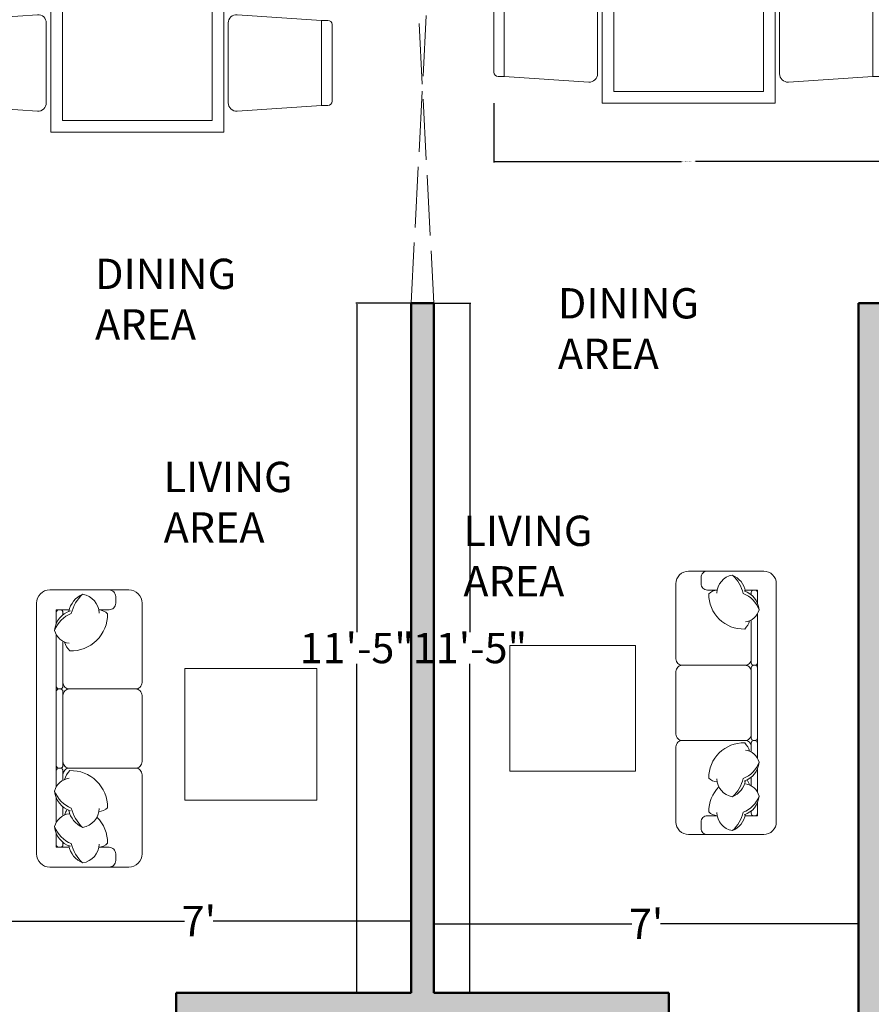
# Model space of a CAD drawing. Units: inches. Extents: x -28 to 544, y -640 to 52.
# Tile 5 of 11: x 169 to 338, y -389 to -194. Entities that reach past the tile are written whole.
import ezdxf

# ---------------------------------------------------------------- set-up
doc = ezdxf.new("R2010")
doc.units = ezdxf.units.IN
doc.header["$MEASUREMENT"] = 0
doc.linetypes.add('ACAD_ISO02W100', pattern=[15, 12, -3])
for name, color, linetype, lineweight in [('A-ANNO-DIMS', 2, 'Continuous', 18), ('A-AREA-IDEN', 7, 'Continuous', 25), ('A-FURN', 8, 'Continuous', 18), ('A-WALL', 7, 'Continuous', 50), ('A-WALL-OVHD', 8, 'ACAD_ISO02W100', 18), ('A-WALL-PATT', 5, 'Continuous', 13)]:
    doc.layers.add(name, color=color, linetype=linetype, lineweight=lineweight)
doc.styles.get("Standard").update_dxf_attribs({"font": 'arial.ttf'})
doc.dimstyles.get("Standard").update_dxf_attribs({"dimtxt": 0.18, "dimasz": 0.18, "dimexe": 0.18, "dimexo": 0.0625, "dimgap": 0.09, "dimtad": 0, "dimtih": 1, "dimtoh": 1, "dimdec": 0, "dimzin": 0, "dimdsep": 46, "dimlunit": 3, "dimtxsty": 'Standard', "dimcen": 0.09, "dimadec": 0, "dimazin": 0, "dimtfac": 1, "dimtdec": 0, "dimtofl": 0, "dimtmove": 0, "dimatfit": 3, "dimfxl": 1, "dimtolj": 1, "dimtzin": 0, "dimarcsym": 0})

# ---------------------------------------------------------------- blocks, each defined once
blk = doc.blocks.new('*D39')
at = {"layer": 'A-ANNO-DIMS', "color": 0, "lineweight": -2, "transparency": 16777216}
for p, q in [((162.44, -377.5), (162.44, -372.33)), ((162.62, -372.51), (201.62, -372.51)), ((246.26, -372.51), (207.27, -372.51)), ((246.44, -377.5), (246.44, -372.33))]:
    blk.add_line(p, q, dxfattribs=at)
at = {"layer": 'A-ANNO-DIMS', "color": 0, "transparency": 16777216}
for points in [[(162.62, -372.48), (162.62, -372.54), (162.44, -372.51)], [(246.26, -372.48), (246.26, -372.54), (246.44, -372.51)]]:
    blk.add_solid(points, dxfattribs=at)
at = {"layer": 'Defpoints', "color": 0, "transparency": 16777216}
for p in [(246.44, -372.51), (162.44, -377.56), (246.44, -377.56)]:
    blk.add_point(p, dxfattribs=at)
at = {"layer": 'A-ANNO-DIMS', "color": 0, "transparency": 16777216, "insert": (204.44, -372.51), "char_height": 6, "attachment_point": 5}
blk.add_mtext("\\A1;7'", dxfattribs=at)
blk = doc.blocks.new('*D40')
at = {"layer": 'A-ANNO-DIMS', "color": 0, "lineweight": -2, "transparency": 16777216}
for p, q in [((250.94, -372.57), (250.94, -373.27)), ((251.12, -373.09), (290.12, -373.09)), ((334.76, -373.09), (295.77, -373.09)), ((334.94, -372.57), (334.94, -373.27))]:
    blk.add_line(p, q, dxfattribs=at)
at = {"layer": 'A-ANNO-DIMS', "color": 0, "transparency": 16777216}
for points in [[(251.12, -373.06), (251.12, -373.12), (250.94, -373.09)], [(334.76, -373.06), (334.76, -373.12), (334.94, -373.09)]]:
    blk.add_solid(points, dxfattribs=at)
at = {"layer": 'Defpoints', "color": 0, "transparency": 16777216}
for p in [(250.94, -372.51), (334.94, -372.51), (334.94, -373.09)]:
    blk.add_point(p, dxfattribs=at)
at = {"layer": 'A-ANNO-DIMS', "color": 0, "transparency": 16777216, "insert": (292.94, -373.09), "char_height": 6, "width": 5.472, "attachment_point": 5}
blk.add_mtext("\\A1;7'", dxfattribs=at)
blk = doc.blocks.new('*D43')
at = {"layer": 'A-ANNO-DIMS', "color": 0, "lineweight": -2, "transparency": 16777216}
for p, q in [((251.01, -250.24), (258.27, -250.24)), ((258.09, -250.42), (258.09, -315.34)), ((258.09, -386.56), (258.09, -321.64)), ((251.01, -386.74), (258.27, -386.74))]:
    blk.add_line(p, q, dxfattribs=at)
at = {"layer": 'A-ANNO-DIMS', "color": 0, "transparency": 16777216}
for points in [[(258.06, -250.42), (258.12, -250.42), (258.09, -250.24)], [(258.06, -386.56), (258.12, -386.56), (258.09, -386.74)]]:
    blk.add_solid(points, dxfattribs=at)
at = {"layer": 'Defpoints', "color": 0, "transparency": 16777216}
for p in [(250.94, -250.24), (250.94, -386.74), (258.09, -386.74)]:
    blk.add_point(p, dxfattribs=at)
at = {"layer": 'A-ANNO-DIMS', "color": 0, "transparency": 16777216, "insert": (258.09, -318.49), "char_height": 6, "attachment_point": 5}
blk.add_mtext('\\A1;11\'-5"', dxfattribs=at)
blk = doc.blocks.new('*D44')
at = {"layer": 'A-ANNO-DIMS', "color": 0, "lineweight": -2, "transparency": 16777216}
for p, q in [((246.38, -250.24), (235.51, -250.24)), ((235.69, -250.42), (235.69, -315.34)), ((235.69, -386.56), (235.69, -321.64)), ((246.38, -386.74), (235.51, -386.74))]:
    blk.add_line(p, q, dxfattribs=at)
at = {"layer": 'A-ANNO-DIMS', "color": 0, "transparency": 16777216}
for points in [[(235.66, -250.42), (235.72, -250.42), (235.69, -250.24)], [(235.66, -386.56), (235.72, -386.56), (235.69, -386.74)]]:
    blk.add_solid(points, dxfattribs=at)
at = {"layer": 'Defpoints', "color": 0, "transparency": 16777216}
for p in [(235.69, -250.24), (246.44, -250.24), (246.44, -386.74)]:
    blk.add_point(p, dxfattribs=at)
at = {"layer": 'A-ANNO-DIMS', "color": 0, "transparency": 16777216, "insert": (235.69, -318.49), "char_height": 6, "attachment_point": 5}
blk.add_mtext('\\A1;11\'-5"', dxfattribs=at)
blk = doc.blocks.new('DINING-SET-4')
for p, q in [((0.82, 49.45), (2.05, 49.45)), ((18.79, 50.59), (2.05, 49.45)), ((2.05, 32.63), (2.05, 49.45)), ((20.52, 48.95), (20.52, 33.13)), ((56.54, 48.95), (56.54, 33.13)), ((58.27, 50.59), (75.01, 49.45)), ((76.24, 49.45), (75.01, 49.45)), ((75.01, 32.63), (75.01, 49.45)), ((0, 33.45), (0, 48.63)), ((77.06, 33.45), (77.06, 48.63)), ((2.05, 32.63), (0.82, 32.63)), ((2.05, 32.63), (18.79, 31.49)), ((75.01, 32.63), (58.27, 31.49)), ((75.01, 32.63), (76.24, 32.63)), ((2.05, 22.09), (0.82, 22.09)), ((2.05, 22.09), (18.79, 23.23)), ((2.05, 22.09), (2.05, 5.27)), ((20.52, 5.77), (20.52, 21.59)), ((56.54, 5.77), (56.54, 21.59)), ((75.01, 22.09), (58.27, 23.23)), ((75.01, 22.09), (76.24, 22.09)), ((75.01, 22.09), (75.01, 5.27)), ((0, 21.27), (0, 6.09)), ((77.06, 21.27), (77.06, 6.09)), ((0.82, 5.27), (2.05, 5.27)), ((18.79, 4.13), (2.05, 5.27)), ((58.27, 4.13), (75.01, 5.27)), ((76.24, 5.27), (75.01, 5.27))]:
    blk.add_line(p, q)
for points in [[(55.63, 0), (21.43, 0), (21.43, 54.72), (55.63, 54.72)], [(53.35, 2.28), (23.71, 2.28), (23.71, 52.44), (53.35, 52.44)]]:
    blk.add_lwpolyline(points, close=True)
for centre, radius, start, end in [((0.82, 48.63), 0.821, 90, 180), ((18.88, 48.95), 1.64, 0, 93.1221), ((58.18, 48.95), 1.64, 86.8779, 180), ((76.24, 48.63), 0.821, 0, 90), ((0.82, 33.45), 0.821, 180, 270), ((18.88, 33.13), 1.64, 266.8779, 0), ((58.18, 33.13), 1.64, 180, 273.1221), ((76.24, 33.45), 0.821, 270, 0), ((0.82, 21.27), 0.821, 90, 180), ((18.88, 21.59), 1.64, 0, 93.1221), ((58.18, 21.59), 1.64, 86.8779, 180), ((76.24, 21.27), 0.821, 0, 90), ((0.82, 6.09), 0.821, 180, 270), ((76.24, 6.09), 0.821, 270, 0), ((18.88, 5.77), 1.64, 266.8779, 0), ((58.18, 5.77), 1.64, 180, 273.1221)]:
    blk.add_arc(centre, radius, start, end)
blk = doc.blocks.new('*D71')
at = {"layer": 'A-ANNO-DIMS', "color": 0, "lineweight": -2, "transparency": 16777216}
for p, q in [((262.82, -210.68), (262.82, -222.36)), ((339.88, -210.68), (339.88, -222.36)), ((263, -222.18), (299.96, -222.18)), ((339.7, -222.18), (302.74, -222.18))]:
    blk.add_line(p, q, dxfattribs=at)
at = {"layer": 'A-ANNO-DIMS', "color": 0, "transparency": 16777216}
for points in [[(263, -222.15), (263, -222.21), (262.82, -222.18)], [(339.7, -222.15), (339.7, -222.21), (339.88, -222.18)]]:
    blk.add_solid(points, dxfattribs=at)
at = {"layer": 'Defpoints', "color": 0, "transparency": 16777216}
for p in [(262.82, -210.62), (339.88, -210.62), (339.88, -222.18)]:
    blk.add_point(p, dxfattribs=at)
at = {"layer": 'A-ANNO-DIMS', "color": 0, "transparency": 16777216, "insert": (301.35, -222.18), "char_height": 0.18, "attachment_point": 5}
blk.add_mtext('\\A1;DINING SET 6\'-5" TYP.', dxfattribs=at)

msp = doc.modelspace()

# ---------------------------------------------------------------- hatches: boundary and pattern name
at = {"layer": 'A-WALL-PATT'}
h = msp.add_hatch(color=256, dxfattribs=at)
h.dxf.hatch_style = 1
h.paths.add_polyline_path([(375.44, 7.76), (310.94, 7.76), (310.94, -1.24), (334.94, -1.24), (334.94, -133.24), (286.94, -133.24), (286.94, -137.74), (342.44, -137.74), (342.44, -133.24), (339.44, -133.24), (339.44, -1.24), (375.44, -1.24)])
h.paths.add_polyline_path([(480.44, 7.76), (435.44, 7.76), (435.44, -1.24), (471.44, -1.24), (471.44, -37.24), (480.44, -37.24)])
h.paths.add_polyline_path([(480.44, -97.24), (471.44, -97.24), (471.44, -133.24), (417.44, -133.24), (417.44, -135.49), (417.44, -137.74), (471.44, -137.74), (471.44, -152.74), (480.44, -152.74)])
h.paths.add_polyline_path([(480.44, -176.74), (471.44, -176.74), (471.44, -191.74), (387.44, -191.74), (387.44, -137.74), (389.44, -137.74), (389.44, -133.24), (370.44, -133.24), (370.44, -135.49), (370.44, -137.74), (382.94, -137.74), (382.94, -191.74), (382.94, -196.24), (382.94, -220.24), (385.19, -220.24), (387.44, -220.24), (387.44, -196.24), (471.44, -196.24), (471.44, -211.24), (480.44, -211.24)])
h.paths.add_polyline_path([(480.44, -235.24), (471.44, -235.24), (471.44, -250.24), (387.44, -250.24), (387.44, -248.24), (382.94, -248.24), (382.94, -250.24), (369.44, -250.24), (369.44, -252.49), (369.44, -254.74), (471.44, -254.74), (471.44, -290.74), (480.44, -290.74)])
h.paths.add_polyline_path([(480.44, -350.74), (471.44, -350.74), (471.44, -386.74), (339.44, -386.74), (339.44, -254.74), (341.44, -254.74), (341.44, -250.24), (334.94, -250.24), (334.94, -391.24), (471.44, -391.24), (471.44, -403.24), (480.44, -403.24)])
h.paths.add_polyline_path([(480.44, -427.24), (471.44, -427.24), (471.44, -439.24), (334.94, -439.24), (334.94, -446.74), (339.44, -446.74), (339.44, -443.74), (471.44, -443.74), (471.44, -481.24), (480.44, -481.24)])
h.paths.add_polyline_path([(480.44, -541.24), (471.44, -541.24), (471.44, -578.74), (435.44, -578.74), (435.44, -587.74), (480.44, -587.74)])
h.paths.add_polyline_path([(375.44, -578.74), (339.44, -578.74), (339.44, -474.74), (337.19, -474.74), (334.94, -474.74), (334.94, -578.74), (296.69, -578.74), (296.69, -587.74), (375.44, -587.74)])
h = msp.add_hatch(color=256, dxfattribs=at)
h.dxf.hatch_style = 1
h.paths.add_polyline_path([(246.44, -386.74), (199.94, -386.74), (199.94, -391.24), (199.94, -523.24), (205.44, -523.24), (205.44, -391.24), (246.44, -391.24), (246.44, -433.24), (250.94, -433.24), (250.94, -391.24), (291.94, -391.24), (291.94, -523.24), (297.44, -523.24), (297.44, -386.74), (250.94, -386.74), (250.94, -250.24), (246.44, -250.24)])
h.paths.add_polyline_path([(244.06, -411.97), (253.32, -411.97), (253.32, -399.6), (244.06, -399.6)], flags=25)

# ---------------------------------------------------------------- linework, layer by layer
at = {"layer": 'A-FURN', "ltscale": 0.03}
for points in [[(301.33, -303.27, 0.414214), (298.85, -305.75), (298.85, -320.65, 0.414214), (300.09, -321.89, 0.414214), (298.85, -323.13), (298.85, -335.54, 0.414214), (300.09, -336.78, 0.414214), (298.85, -338.02), (298.85, -352.92, 0.414214), (301.33, -355.4), (316.23, -355.4, 0.414214), (318.71, -352.92), (318.71, -305.75, 0.414214), (316.23, -303.27)], [(190.6, -306.99, -0.414214), (193.21, -309.61), (193.21, -325.28, -0.414214), (191.91, -326.58, -0.414214), (193.21, -327.89), (193.21, -340.95, -0.414214), (191.91, -342.25, -0.414214), (193.21, -343.56), (193.21, -359.23, -0.414214), (190.6, -361.84), (174.93, -361.84, -0.414214), (172.32, -359.23), (172.32, -309.61, -0.414214), (174.93, -306.99)]]:
    msp.add_lwpolyline(points, format="xyb", close=True, dxfattribs=at)
at = {"layer": 'A-FURN'}
for points in [[(305.06, -303.27, 0.414214), (303.82, -304.51), (303.82, -305.75, 0.414214), (305.06, -307), (306.98, -307)], [(306.91, -307.62, -0.356772), (310.03, -304.06, -0.249542), (312.61, -307.28, 9.61688)], [(310.03, -304.06, -0.14773), (312.17, -307.69, -0.213343), (315.3, -310.89, -0.178662)], [(181.45, -307.83, 0.14773), (179.2, -311.64, 0.213343), (175.91, -315.01, 0.178662)], [(184.74, -311.57, 0.356772), (181.45, -307.83, 0.249542), (178.73, -311.22, -9.61688)], [(186.68, -306.99, -0.414214), (187.99, -308.3), (187.99, -309.61, -0.414214), (186.68, -310.91), (184.66, -310.91)], [(306.98, -306.99, 0.165541), (305.34, -307.76, 0.425989), (312.45, -314.73, 0.121523), (313.43, -313.08, -7.115464)], [(312.34, -307.19, -0.306663), (315.3, -310.89, -0.30633), (312.59, -313.31, 0.872847)], [(313.75, -307.94), (313.75, -307.49, -0.414214), (314.24, -307), (314.49, -307, -0.414214), (314.99, -307.49)], [(314.99, -307.49), (314.99, -309.61, -0.414214)], [(179.02, -311.11, 0.306663), (175.91, -315.01, 0.30633), (178.75, -317.55, -0.872847)], [(177.54, -311.91), (177.54, -311.43, 0.414214), (177.02, -310.91), (176.76, -310.91, 0.414214), (176.24, -311.43)], [(176.24, -311.43), (176.24, -313.66, 0.414214)], [(184.66, -310.91, -0.165541), (186.38, -311.72, -0.425989), (178.9, -319.05, -0.121523), (177.87, -317.31, 7.115464)], [(314.99, -311.67), (314.99, -321.39, -0.414214), (314.49, -321.89), (314.24, -321.89, -0.414214), (313.75, -321.39), (313.75, -312.92, -0.414214)], [(176.24, -315.83), (176.24, -326.06, 0.414214), (176.76, -326.58), (177.02, -326.58, 0.414214), (177.54, -326.06), (177.54, -317.15, 0.414214)], [(313.75, -320.65, -0.414214), (312.5, -321.89), (300.09, -321.89, -0.414214)], [(313.75, -323.13, 0.414214), (312.5, -321.89)], [(177.54, -325.28, 0.414214), (178.85, -326.58), (191.91, -326.58, 0.414214)], [(177.54, -327.89, -0.414214), (178.85, -326.58)], [(313.75, -338.02, 0.414214), (312.5, -336.78), (300.09, -336.78, 0.414214)], [(313.75, -335.54, -0.414214), (312.5, -336.78)], [(314.99, -340.31), (314.99, -337.28, 0.414214), (314.49, -336.78), (314.24, -336.78, 0.414214), (313.75, -337.28), (313.75, -339.07, 0.414214)], [(306.98, -344.99, -0.165541), (305.34, -344.23, -0.425989), (312.45, -337.26, -0.121523), (313.43, -338.91, 7.115464)], [(312.34, -344.8, 0.306663), (315.3, -341.1, 0.30633), (312.59, -338.68, -0.872847)], [(177.54, -340.95, 0.414214), (178.85, -342.25)], [(176.24, -345.97), (176.24, -342.78, -0.414214), (176.76, -342.25), (177.02, -342.25, -0.414214), (177.54, -342.78), (177.54, -344.65, -0.414214)], [(177.54, -343.56, -0.414214), (178.85, -342.25), (191.91, -342.25, -0.414214)], [(184.66, -350.89, 0.165541), (186.38, -350.08, 0.425989), (178.9, -342.75, 0.121523), (177.87, -344.49, -7.115464)], [(310.03, -347.92, 0.14773), (312.17, -344.3, 0.213343), (315.3, -341.1, 0.178662)], [(314.99, -347), (314.99, -342.38, 0.414214)], [(179.02, -350.69, -0.306663), (175.91, -346.79, -0.30633), (178.75, -344.25, 0.872847)], [(306.91, -344.37, 0.356772), (310.03, -347.92, 0.249542), (312.61, -344.7, -9.61688)], [(312.95, -344.56, -0.071865), (313.43, -345.6, 7.115464)], [(313.75, -344.04), (313.75, -345.75, 0.414214)], [(181.45, -353.98, -0.14773), (179.2, -350.16, -0.213343), (175.91, -346.79, -0.178662)], [(306.98, -351.68, -0.165541), (305.34, -350.91, -0.200231), (307.34, -345.98, -0.121523)], [(312.34, -351.48, 0.306663), (315.3, -347.78, 0.30633), (312.59, -345.36, -0.872847)], [(176.24, -353), (176.24, -348.14, -0.414214)], [(310.03, -354.61, 0.14773), (312.17, -350.98, 0.213343), (315.3, -347.78, 0.178662)], [(177.54, -349.89), (177.54, -351.69, -0.414214)], [(178.38, -350.43, 0.071865), (177.87, -351.53, -7.115464)], [(184.74, -350.23, -0.356772), (181.45, -353.98, -0.249542), (178.73, -350.58, 9.61688)], [(314.99, -349.07), (314.99, -351.68), (312.55, -351.68, 0.414214)], [(313.75, -350.73), (313.75, -351.18, 0.414214), (314.24, -351.68), (314.49, -351.68, 0.414214), (314.99, -351.18)], [(314.99, -351.18), (314.99, -349.07, 0.414214)], [(179.02, -357.72, -0.306663), (175.91, -353.83, -0.30633), (178.75, -351.28, 0.872847)], [(184.66, -357.93, 0.165541), (186.38, -357.12, 0.200231), (184.28, -351.93, 0.121523)], [(306.98, -351.68), (305.06, -351.68, 0.414214), (303.82, -352.92), (303.82, -354.16, 0.414214), (305.06, -355.4)], [(306.91, -351.05, 0.356772), (310.03, -354.61, 0.249542), (312.61, -351.39, -9.61688)], [(181.45, -361.01, -0.14773), (179.2, -357.19, -0.213343), (175.91, -353.83, -0.178662)], [(176.24, -355.18), (176.24, -357.92), (178.8, -357.92, -0.414214)], [(176.24, -357.4), (176.24, -355.18, -0.414214)], [(177.54, -356.93), (177.54, -357.4, -0.414214), (177.02, -357.92), (176.76, -357.92, -0.414214), (176.24, -357.4)], [(184.74, -357.27, -0.356772), (181.45, -361.01, -0.249542), (178.73, -357.62, 9.61688)], [(184.66, -357.92), (186.68, -357.92, -0.414214), (187.99, -359.23), (187.99, -360.54, -0.414214), (186.68, -361.84)]]:
    msp.add_lwpolyline(points, format="xyb", dxfattribs=at)
for points in [[(312.55, -307), (314.99, -307), (314.99, -309.61)], [(178.8, -310.91), (176.24, -310.91), (176.24, -313.66)], [(314.99, -311.67), (314.99, -340.31)], [(176.24, -315.83), (176.24, -345.97)], [(314.99, -342.38), (314.99, -347)], [(176.24, -348.14), (176.24, -353)]]:
    msp.add_lwpolyline(points, dxfattribs=at)
at = {"layer": 'A-FURN', "ltscale": 0.03}
for points in [[(266, -342.83), (266, -318.01), (290.82, -318.01), (290.82, -342.83)], [(227.78, -348.62), (227.78, -322.5), (201.66, -322.5), (201.66, -348.62)]]:
    msp.add_lwpolyline(points, close=True, dxfattribs=at)
at = {"layer": 'A-FURN'}
for points in [[(314.99, -336.29), (314.99, -322.39, 0.414214), (314.49, -321.89), (314.24, -321.89, 0.414214), (313.75, -322.39), (313.75, -336.29, 0.414214), (314.24, -336.78), (314.49, -336.78, 0.414214)], [(176.24, -341.73), (176.24, -327.1, -0.414214), (176.76, -326.58), (177.02, -326.58, -0.414214), (177.54, -327.1), (177.54, -341.73, -0.414214), (177.02, -342.25), (176.76, -342.25, -0.414214)]]:
    msp.add_lwpolyline(points, format="xyb", close=True, dxfattribs=at)
at = {"layer": 'A-WALL'}
for p, q in [((246.44, -250.24), (250.94, -250.24)), ((246.44, -250.24), (246.44, -386.74)), ((250.94, -250.24), (250.94, -386.74)), ((334.94, -250.24), (341.44, -250.24)), ((334.94, -250.24), (334.94, -391.24)), ((246.44, -386.74), (199.94, -386.74)), ((199.94, -386.74), (199.94, -386.74)), ((199.94, -391.24), (199.94, -386.74)), ((297.44, -386.74), (250.94, -386.74)), ((297.44, -523.24), (297.44, -386.74))]:
    msp.add_line(p, q, dxfattribs=at)
at = {"layer": 'A-WALL-OVHD'}
for p, q in [((246.44, -164.95), (250.94, -250.24)), ((246.44, -250.24), (250.94, -164.95))]:
    msp.add_line(p, q, dxfattribs=at)

# ---------------------------------------------------------------- block references
at = {"layer": 'A-FURN'}
for p in [(262.82, -210.62), (153.73, -216.37)]:
    msp.add_blockref('DINING-SET-4', p, dxfattribs=at)

# ---------------------------------------------------------------- texts
at = {"layer": 'A-AREA-IDEN', "insert": (183.91, -241.43), "char_height": 6, "attachment_point": 1}
msp.add_mtext_dynamic_manual_height_columns('DINING\\PAREA', width=1.7957, gutter_width=1, heights=[0], dxfattribs=at)
at = {"layer": 'A-AREA-IDEN', "char_height": 6, "attachment_point": 1}
for s, insert in [('DINING \\PAREA', (275.49, -247.26)), ('LIVING\\PAREA', (197.47, -281.63)), ('LIVING \\PAREA', (256.79, -292.28))]:
    msp.add_mtext(s, dxfattribs=dict(at, insert=insert))

# ---------------------------------------------------------------- dimensions: what is measured, and where the dimension line sits
at = {"layer": 'A-ANNO-DIMS'}
dim = msp.add_linear_dim(base=(339.88, -222.18), p1=(262.82, -210.62), p2=(339.88, -210.62), text='DINING SET <> TYP.', dimstyle='Standard', override={"dimdec": 1, "dimlfac": 1, "dimrnd": 0, "dimzin": 1, "dimdsep": 46, "dimlunit": 4, "dimfrac": 2}, dxfattribs=at)
dim.commit()
dim.dimension.update_dxf_attribs({"geometry": '*D71', "text_midpoint": (301.35, -222.18)})
for base, p1, p2, picture, middle in [((235.69210062, -250.24117838), (246.44473605, -386.74117838), (246.44473605, -250.24117838), '*D44', (235.69210062, -318.49117838)), ((258.08966266, -386.74117838), (250.94473605, -250.24117838), (250.94473605, -386.74117838), '*D43', (258.08966266, -318.49117838))]:
    dim = msp.add_linear_dim(base=base, p1=p1, p2=p2, angle=90, dimstyle='Standard', override={"dimtxt": 6, "dimclrd": 0, "dimclre": 0, "dimclrt": 0}, dxfattribs=at)
    dim.commit()
    dim.dimension.update_dxf_attribs({"geometry": picture, "text_midpoint": middle})
for base, p1, p2, picture, middle in [((246.44, -372.51), (162.44, -377.56), (246.44, -377.56), '*D39', (204.44, -372.51)), ((334.94, -373.09), (250.94, -372.51), (334.94, -372.51), '*D40', (292.94, -373.09))]:
    dim = msp.add_linear_dim(base=base, p1=p1, p2=p2, dimstyle='Standard', override={"dimtxt": 6, "dimclrd": 0, "dimclre": 0, "dimclrt": 0}, dxfattribs=at)
    dim.commit()
    dim.dimension.update_dxf_attribs({"geometry": picture, "text_midpoint": middle})

doc.saveas('drawing.dxf')
